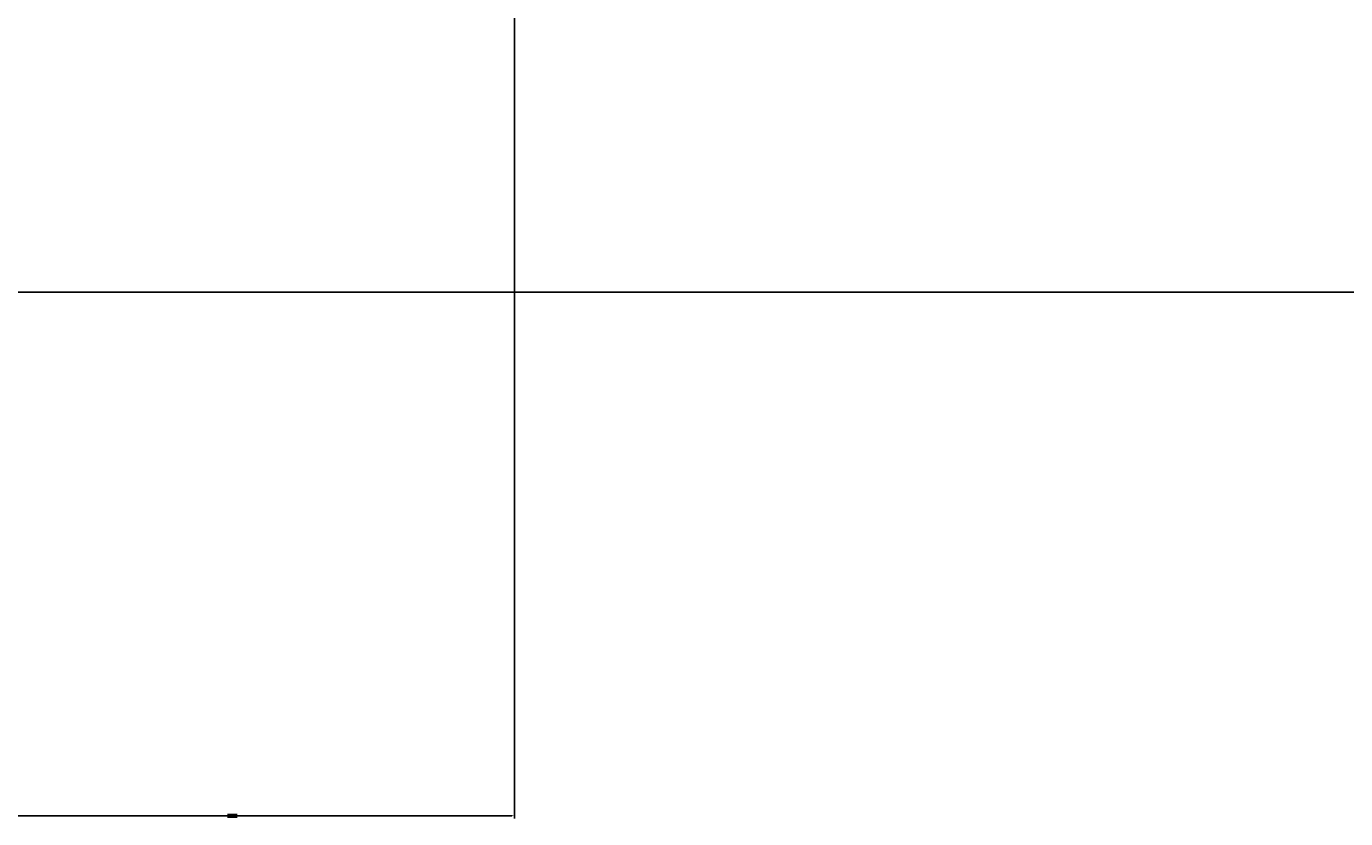
# Model space of a CAD drawing. Units: inches. Extents: x -301 to 715, y -607 to 364.
# Tile 13 of 141: x 18 to 101, y -574 to -524. Entities that reach past the tile are written whole.
import ezdxf

# ---------------------------------------------------------------- set-up
doc = ezdxf.new("R2010")
doc.units = ezdxf.units.IN
doc.header["$MEASUREMENT"] = 0
doc.layers.add('A-ANNO-DIMS', color=2, linetype='Continuous', lineweight=18)
doc.styles.get("Standard").update_dxf_attribs({"font": 'arial.ttf'})
doc.dimstyles.get("Standard").update_dxf_attribs({"dimtxt": 0.18, "dimasz": 0.18, "dimexe": 0.18, "dimexo": 0.0625, "dimgap": 0.09, "dimtad": 0, "dimtih": 1, "dimtoh": 1, "dimdec": 1, "dimzin": 0, "dimdsep": 46, "dimlunit": 4, "dimtxsty": 'Standard', "dimcen": 0.09, "dimclrd": 3, "dimclre": 4, "dimclrt": 6, "dimadec": 0, "dimazin": 0, "dimtfac": 1, "dimtdec": 1, "dimtofl": 0, "dimtmove": 0, "dimatfit": 3, "dimfxl": 1, "dimtfill": 2, "dimtfillclr": 51, "dimtolj": 1, "dimtzin": 0, "dimarcsym": 0})

# ---------------------------------------------------------------- blocks, each defined once
blk = doc.blocks.new('*D176')
at = {"layer": 'A-ANNO-DIMS', "color": 4, "lineweight": -2, "transparency": 16777216}
for p, q in [((148.28, -324.477), (215.605, -324.477)), ((-15.22, -540.477), (215.605, -540.477))]:
    blk.add_line(p, q, dxfattribs=at)
at = {"layer": 'A-ANNO-DIMS', "color": 3, "lineweight": -2, "transparency": 16777216}
for p, q in [((215.425, -324.657), (215.425, -432.296)), ((215.425, -540.297), (215.425, -432.659))]:
    blk.add_line(p, q, dxfattribs=at)
at = {"layer": 'A-ANNO-DIMS', "color": 3, "transparency": 16777216}
for points in [[(215.395, -324.657), (215.455, -324.657), (215.425, -324.477)], [(215.395, -540.297), (215.455, -540.297), (215.425, -540.477)]]:
    blk.add_solid(points, dxfattribs=at)
at = {"layer": 'Defpoints', "color": 0, "transparency": 16777216}
for p in [(148.218, -324.477), (-15.282, -540.477), (215.425, -540.477)]:
    blk.add_point(p, dxfattribs=at)
at = {"layer": 'A-ANNO-DIMS', "color": 6, "transparency": 16777216, "insert": (215.425, -432.477), "char_height": 0.18, "attachment_point": 5, "bg_fill": 1, "box_fill_scale": 1.25, "bg_fill_color": 51, "bg_fill_transparency": 0}
blk.add_mtext('\\A1;18\'-0"', dxfattribs=at)
blk = doc.blocks.new('*D181')
at = {"layer": 'A-ANNO-DIMS', "color": 4, "lineweight": -2, "transparency": 16777216}
for p, q in [((48.468, -433.54), (48.468, -573.809)), ((12.718, -463.54), (12.718, -573.809))]:
    blk.add_line(p, q, dxfattribs=at)
at = {"layer": 'A-ANNO-DIMS', "color": 3, "lineweight": -2, "transparency": 16777216}
for p, q in [((12.898, -573.629), (30.264, -573.629)), ((48.288, -573.629), (30.922, -573.629))]:
    blk.add_line(p, q, dxfattribs=at)
at = {"layer": 'A-ANNO-DIMS', "color": 3, "transparency": 16777216}
for points in [[(12.898, -573.599), (12.898, -573.659), (12.718, -573.629)], [(48.288, -573.599), (48.288, -573.659), (48.468, -573.629)]]:
    blk.add_solid(points, dxfattribs=at)
at = {"layer": 'Defpoints', "color": 0, "transparency": 16777216}
for p in [(48.468, -433.477), (12.718, -463.477), (48.468, -573.629)]:
    blk.add_point(p, dxfattribs=at)
at = {"layer": 'A-ANNO-DIMS', "color": 6, "transparency": 16777216, "insert": (30.593, -573.629), "char_height": 0.18, "attachment_point": 5, "bg_fill": 1, "box_fill_scale": 1.25, "bg_fill_color": 51, "bg_fill_transparency": 0}
blk.add_mtext('\\A1;3\'-0"', dxfattribs=at)
blk = doc.blocks.new('*D191')
at = {"layer": 'A-ANNO-DIMS', "color": 4, "lineweight": -2, "transparency": 16777216}
for p, q in [((129.193, -481.477), (-266.112, -481.477)), ((114.193, -540.477), (-266.112, -540.477))]:
    blk.add_line(p, q, dxfattribs=at)
at = {"layer": 'A-ANNO-DIMS', "color": 3, "lineweight": -2, "transparency": 16777216}
for p, q in [((-265.932, -481.657), (-265.932, -510.797)), ((-265.932, -540.297), (-265.932, -511.158))]:
    blk.add_line(p, q, dxfattribs=at)
at = {"layer": 'A-ANNO-DIMS', "color": 3, "transparency": 16777216}
for points in [[(-265.962, -481.657), (-265.902, -481.657), (-265.932, -481.477)], [(-265.962, -540.297), (-265.902, -540.297), (-265.932, -540.477)]]:
    blk.add_solid(points, dxfattribs=at)
at = {"layer": 'Defpoints', "color": 0, "transparency": 16777216}
for p in [(129.255, -481.477), (-265.932, -540.477), (114.255, -540.477)]:
    blk.add_point(p, dxfattribs=at)
at = {"layer": 'A-ANNO-DIMS', "color": 6, "transparency": 16777216, "insert": (-265.932, -510.977), "char_height": 0.18, "attachment_point": 5, "bg_fill": 1, "box_fill_scale": 1.25, "bg_fill_color": 51, "bg_fill_transparency": 0}
blk.add_mtext('\\A1;4\'-11"', dxfattribs=at)

msp = doc.modelspace()

# ---------------------------------------------------------------- dimensions: what is measured, and where the dimension line sits
at = {"layer": 'A-ANNO-DIMS'}
for base, p1, p2, picture, middle in [((215.425, -540.477), (148.218, -324.477), (-15.282, -540.477), '*D176', (215.425, -432.477)), ((-265.932, -540.477), (129.255, -481.477), (114.255, -540.477), '*D191', (-265.932, -510.977))]:
    dim = msp.add_linear_dim(base=base, p1=p1, p2=p2, angle=90, dimstyle='Standard', override={"dimdec": 1, "dimlfac": 1, "dimrnd": 0, "dimzin": 1, "dimdsep": 46, "dimlunit": 4, "dimfrac": 2}, dxfattribs=at)
    dim.commit()
    dim.dimension.update_dxf_attribs({"geometry": picture, "text_midpoint": middle})
dim = msp.add_linear_dim(base=(48.467984, -573.628877), p1=(12.717984, -463.47741), p2=(48.467984, -433.47741), dimstyle='Standard', override={"dimdec": 1, "dimlfac": 1, "dimrnd": 0, "dimzin": 1, "dimdsep": 46, "dimlunit": 4, "dimfrac": 2}, dxfattribs=at)
dim.commit()
dim.dimension.update_dxf_attribs({"geometry": '*D181', "text_midpoint": (30.592984, -573.628877)})

doc.saveas('drawing.dxf')
